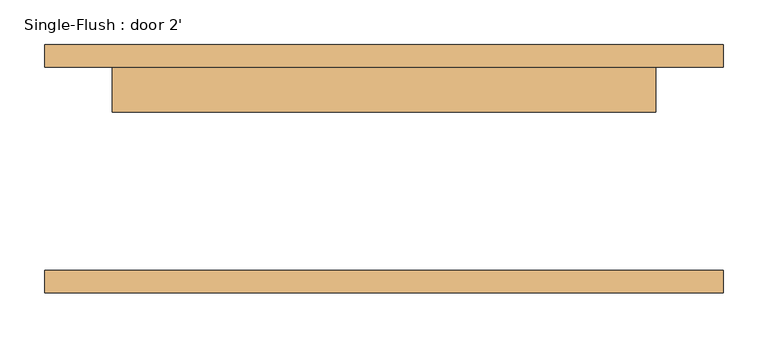
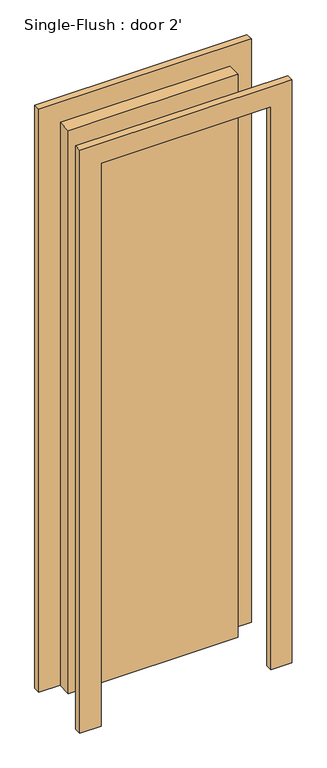
"""IFC4 building model written with IfcOpenShell, lengths in millimetres: door geometry, Single-Flush : door 2'."""

from ifc_helpers import new_model, si_unit, frame, origin, origin_with_axes, place, context, project, spatial, polyline, outline, extrude, source, transform, mapped, element, save


def single_flush_door_2_0d3b4037(model_context):
    return source(origin(), model_context, "Body", "SweptSolid", [
        extrude(outline(polyline([(2209.8, -381.0), (0.0, -381.0), (0.0, -304.8), (2133.6, -304.8), (2133.6, 304.8), (0.0, 304.8), (0.0, 381.0), (2209.8, 381.0), (2209.8, -381.0)])), frame((0.0, 114.3, 0.0), z_axis=(0.0, 1.0, 0.0), x_axis=(0.0, 0.0, 1.0)), (0.0, 0.0, 1.0), 25.4),
        extrude(outline(polyline([(2209.8, 381.0), (2209.8, -381.0), (0.0, -381.0), (0.0, -304.8), (2133.6, -304.8), (2133.6, 304.8), (0.0, 304.8), (0.0, 381.0), (2209.8, 381.0)])), frame((0.0, -139.7, 0.0), z_axis=(0.0, 1.0, 0.0), x_axis=(0.0, 0.0, 1.0)), (0.0, 0.0, 1.0), 25.4),
        extrude(outline(polyline([(304.8, 63.5), (-304.8, 63.5), (-304.8, 114.3), (304.8, 114.3), (304.8, 63.5)])), origin_with_axes(), (0.0, 0.0, 1.0), 2133.6),
    ])


if __name__ == "__main__":
    model = new_model("IFC4")
    model_context = context("Model", 3, world=origin())
    ifc_project = project(units=[si_unit("LENGTHUNIT", "METRE", prefix="MILLI")], contexts=[model_context])
    site = spatial("IfcSite", under=ifc_project)
    building = spatial("IfcBuilding", under=site)
    placement = place(None, origin())
    single_flush_door_2_shape = single_flush_door_2_0d3b4037(model_context)
    element("IfcDoor", 1, ObjectType="Single-Flush : door 2'", at=placement, inside=building, context=model_context, shape_type="MappedRepresentation", body=[
        mapped(single_flush_door_2_shape, transform((0.0, 0.0, 0.0), x_axis=(1.0, 0.0, 0.0), y_axis=(0.0, 1.0, 0.0), z_axis=(0.0, 0.0, 1.0))),
    ])
    save(model, "model.ifc")

# Revit data of these elements
# Type "Single-Flush : door 2'"
#   Type Mark = "11"
#   Construction Type Id = "MDOOR"
#   Assembly Code = "C1020"
#   Analytic Construction = "Metal"
#   Thickness = 0' - 2"
#   Heat Transfer Coefficient (U) = 0.651978 BTU/(h·ft²·°F)
#   Height = 7' - 0"
#   Trim Projection Ext = 0' - 1"
#   Trim Projection Int = 0' - 1"
#   Trim Width = 0' - 3"
#   Width = 2' - 0"
#   Define Thermal Properties by = 1
#   Door Material = Door - Panel
#   Frame Material = Door - Frame
#   Visual Light Transmittance = 0
#   Solar Heat Gain Coefficient = 0
#   Function = (empty or 0)
#   Wall Closure = (empty or 0)
# Element 1 (IfcDoor, "Single-Flush : door 2'")
#   Materials on its faces: "Door - Frame", "Door - Panel"
# Materials
#   "Door - Panel": class "Wood", colour RGB 210 159 95, transparency 0, Cost = 0
#   "Door - Frame": colour RGB 118 70 51, transparency 0, Cost = 0
